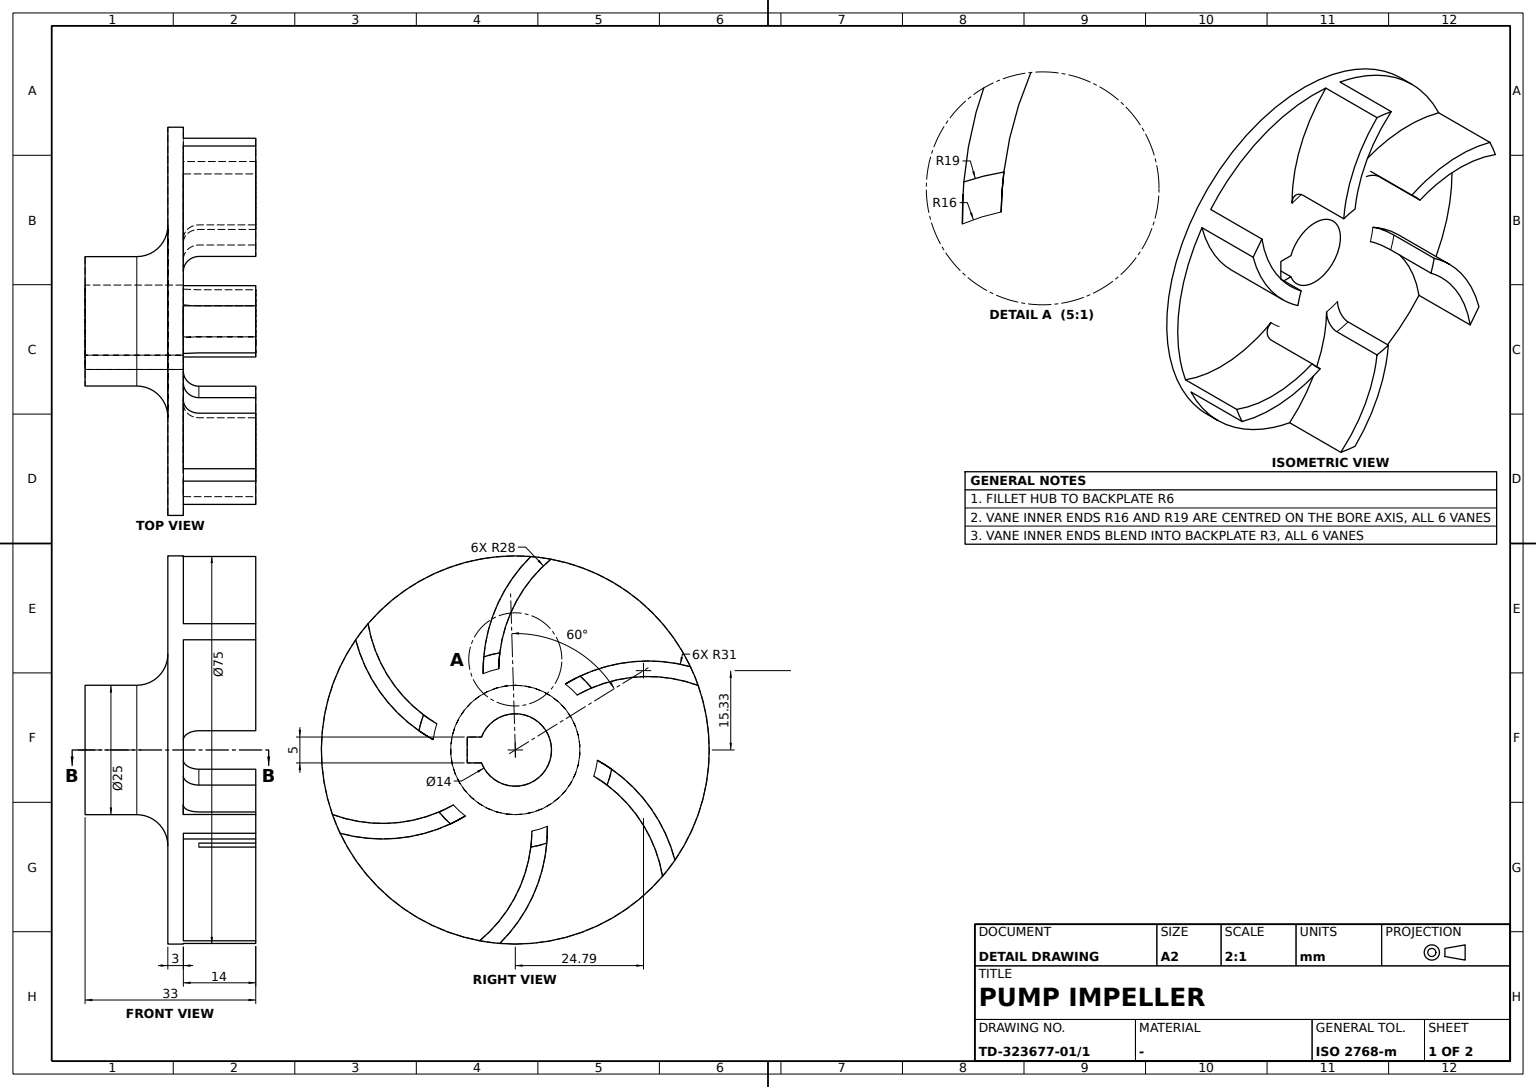
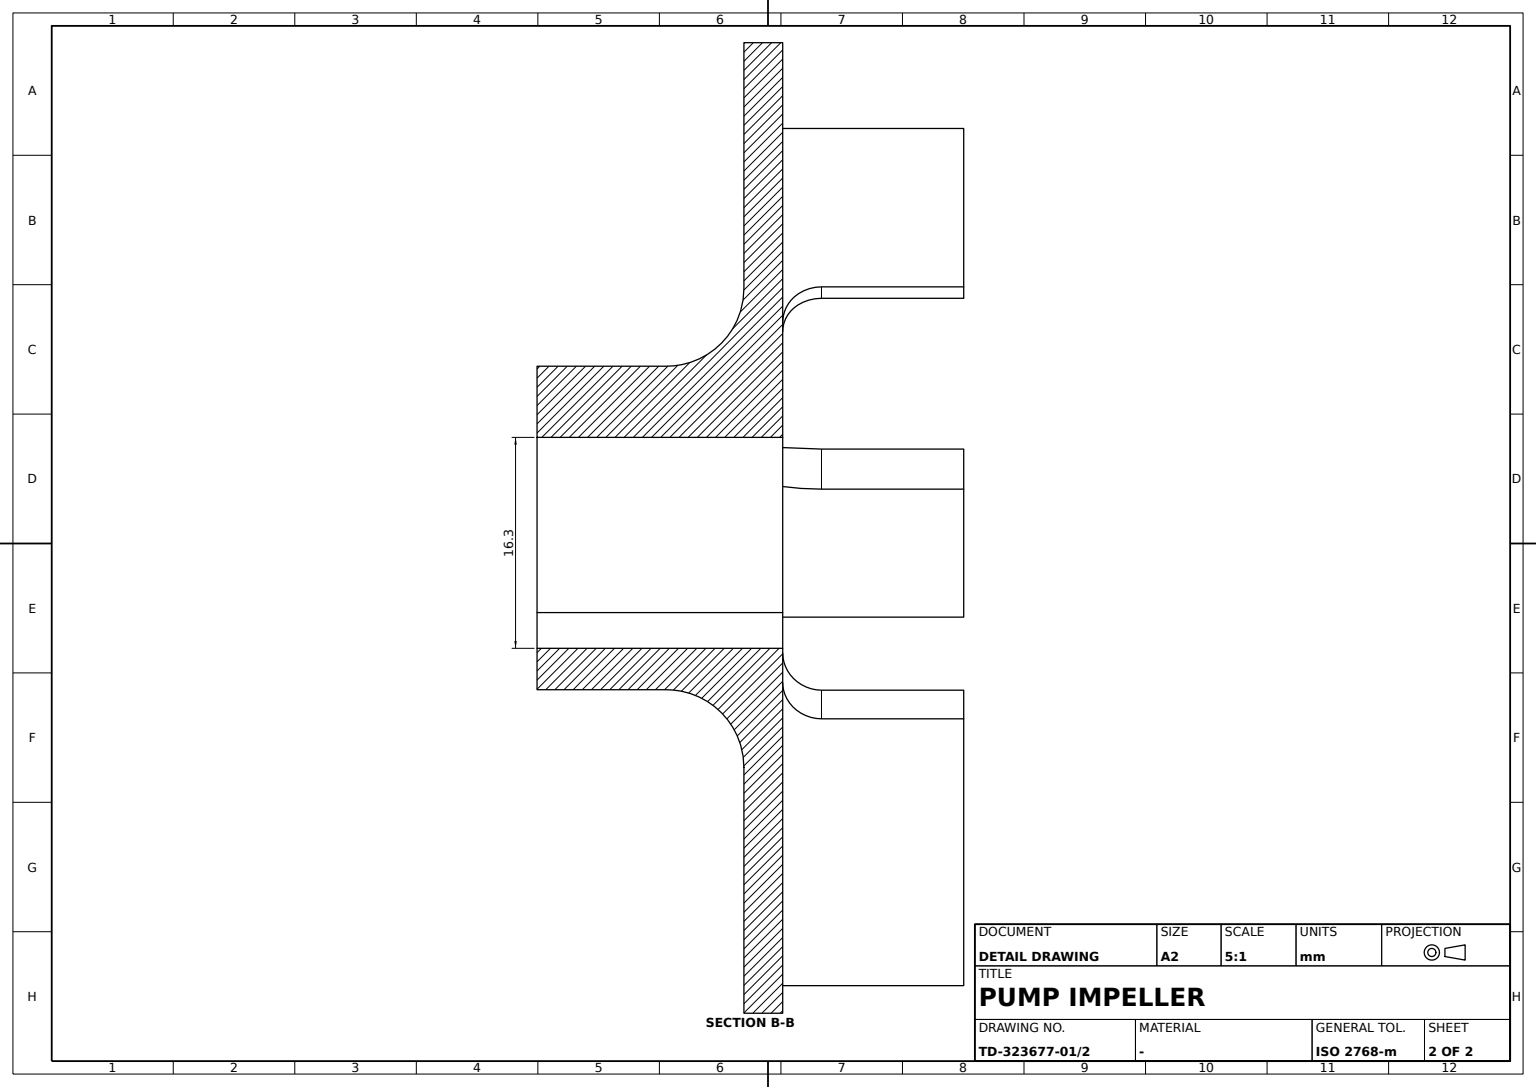
CATIA V5 part; units mm, degrees
sketch "Sketch1" plane through (0, 0, 0) normal (0, 0, 1) x (1, 0, 0)
  circle A0 centre (0, 0) radius 37.5
  dimension "radius A0" = 37.5
extrude "Pad1" add sketch "Sketch1" along normal blind 3
sketch "Sketch2" plane through (0, 0, 3) normal (0, 0, 1) x (1, 0, 0)
  circle A0 centre (0, 0) radius 37.5 construction
  arc A1 (-36.8615, 6.8907) -> (-37.3798, 3) centre (0, 0) ccw
  arc A2 (-37.3798, 3) -> (-17.9954, -6.0963) centre (-15.3287, 24.7888) ccw
  arc A3 (-18.7617, -3) -> (-17.9954, -6.0963) centre (0, 0) ccw
  line L0 (-40.368, 0) -> (58.3834, 0) construction
  point P0 (-40.368, 0)
  line L1 (0, 48.4998) -> (0, -45.6567) construction
  point P1 (0, 48.4998)
  arc A4 (-36.8615, 6.8907) -> (-18.7617, -3) centre (-15.3287, 24.7888) ccw
  point P2 (-15.3287, 24.7888)
  point P3 (-37.3798, 3)
  point P4 (-36.8615, 6.8907)
  point P5 (-18.7617, -3)
  dimension "radius A3" = 19
  dimension "radius A2" = 31
  dimension "radius A4" = 28
  dimension "distance P5 L0" = 3
  dimension "distance P3 L0" = 3
  constraint coincidence P0 x-axis
  constraint coincidence P1 y-axis
  constraint coincidence A0 P3
  constraint coincidence A0 P4
  constraint horizontal L0 x-axis
  constraint vertical L1 y-axis
  constraint concentricity P2 A2
extrude "Pad2" add sketch "Sketch2" along normal blind 14
pattern_circular "CircPattern1" count 6 over 360 about axis through (0, 0, 3) along (0, 0, 1) of "Pad2"
fillet "Fillet1" radius 3 1 edges at (18.4436, 4.5643, 3)
fillet "Fillet2" radius 3 1 edges at (13.1746, -13.6905, 3)
fillet "Fillet3" radius 3 1 edges at (5.2691, 18.2548, 3)
fillet "Fillet4" radius 3 3 edges at (-5.2691, -18.2548, 3) (-18.4436, -4.5643, 3) (-13.1746, 13.6905, 3)
sketch "Sketch3" plane through (0, 0, 0) normal (0, 0, -1) x (1, 0, 0)
  circle A0 centre (0, 0) radius 12.5
  dimension "radius A0" = 12.5
extrude "Pad3" add sketch "Sketch3" along normal blind 16
sketch "Sketch4" plane through (0, 0, -16) normal (0, 0, -1) x (1, 0, 0)
  arc A0 (-2.5, 6.5383) -> (2.5, 6.5383) centre (0, 0) ccw
  line L0 (-2.5, 9.3) -> (2.5, 9.3)
  line L1 (2.5, 9.3) -> (2.5, 6.5383)
  line L2 (-2.5, 6.5383) -> (-2.5, 9.3)
  circle A1 centre (0, 0) radius 12.5 construction
  dimension "radius A0" = 7
  dimension "distance A0 L0" = 16.3
  dimension "length L0" = 5
  dimension "distance L2 y axis" = 2.5
  constraint horizontal L0 x-axis
  constraint vertical L1 y-axis
  constraint vertical L2 y-axis
  constraint concentricity A1 A0
extrude "Pocket1" cut sketch "Sketch4" against normal blind 51
fillet "Fillet5" radius 6 1 edges at (-12.5, 0, 0)
